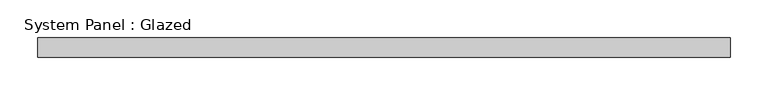
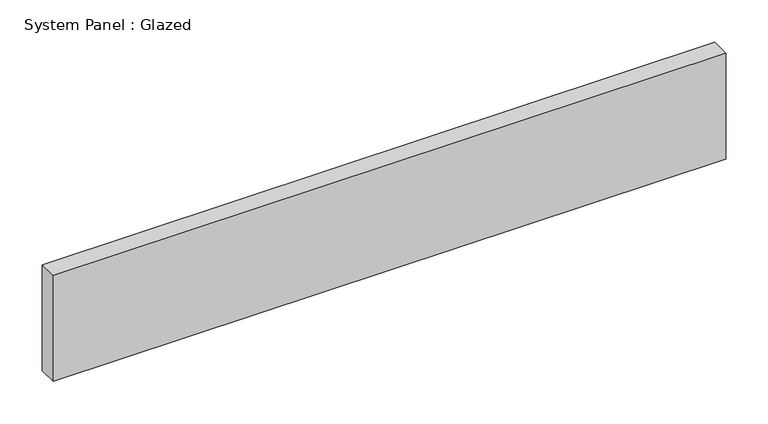
"""IFC4 building model written with IfcOpenShell, lengths in millimetres: plate geometry, System Panel : Glazed."""

from ifc_helpers import new_model, si_unit, origin, origin_with_axes, place, context, project, spatial, polyline, outline, extrude, source, transform, mapped, element, save


def system_panel_glazed_450ffc3c(model_context):
    return source(origin(), model_context, "Body", "SweptSolid", [
        extrude(outline(polyline([(457.2, 19.05), (-457.2, 19.05), (-457.2, 44.45), (457.2, 44.45), (457.2, 19.05)])), origin_with_axes(), (0.0, 0.0, 1.0), 152.4),
    ])


if __name__ == "__main__":
    model = new_model("IFC4")
    model_context = context("Model", 3, world=origin())
    ifc_project = project(units=[si_unit("LENGTHUNIT", "METRE", prefix="MILLI")], contexts=[model_context])
    site = spatial("IfcSite", under=ifc_project)
    building = spatial("IfcBuilding", under=site)
    placement = place(None, origin())
    system_panel_glazed_shape = system_panel_glazed_450ffc3c(model_context)
    element("IfcPlate", 1, ObjectType="System Panel : Glazed", at=placement, inside=building, context=model_context, shape_type="MappedRepresentation", body=[
        mapped(system_panel_glazed_shape, transform((0.0, 0.0, 0.0), x_axis=(1.0, 0.0, 0.0), y_axis=(0.0, 1.0, 0.0), z_axis=(0.0, 0.0, 1.0))),
    ])
    save(model, "model.ifc")

# Revit data of these elements
# Type "System Panel : Glazed"
#   Construction Type Id = "GSP4R"
#   Analytic Construction = "1/8 in Pilkington single glazing"
#   Visual Light Transmittance = 0.9
#   Solar Heat Gain Coefficient = 0.86
#   Heat Transfer Coefficient (U) = 1.18115 BTU/(h·ft²·°F)
#   Define Thermal Properties by = 1
# Element 1 (IfcPlate, "System Panel : Glazed")
#   Materials on its faces: "Glass"
# Materials
#   "Glass": class "Glass", colour RGB 0 128 192, transparency 0.75, Description = "Soda Lime Glass", Cost = 0
